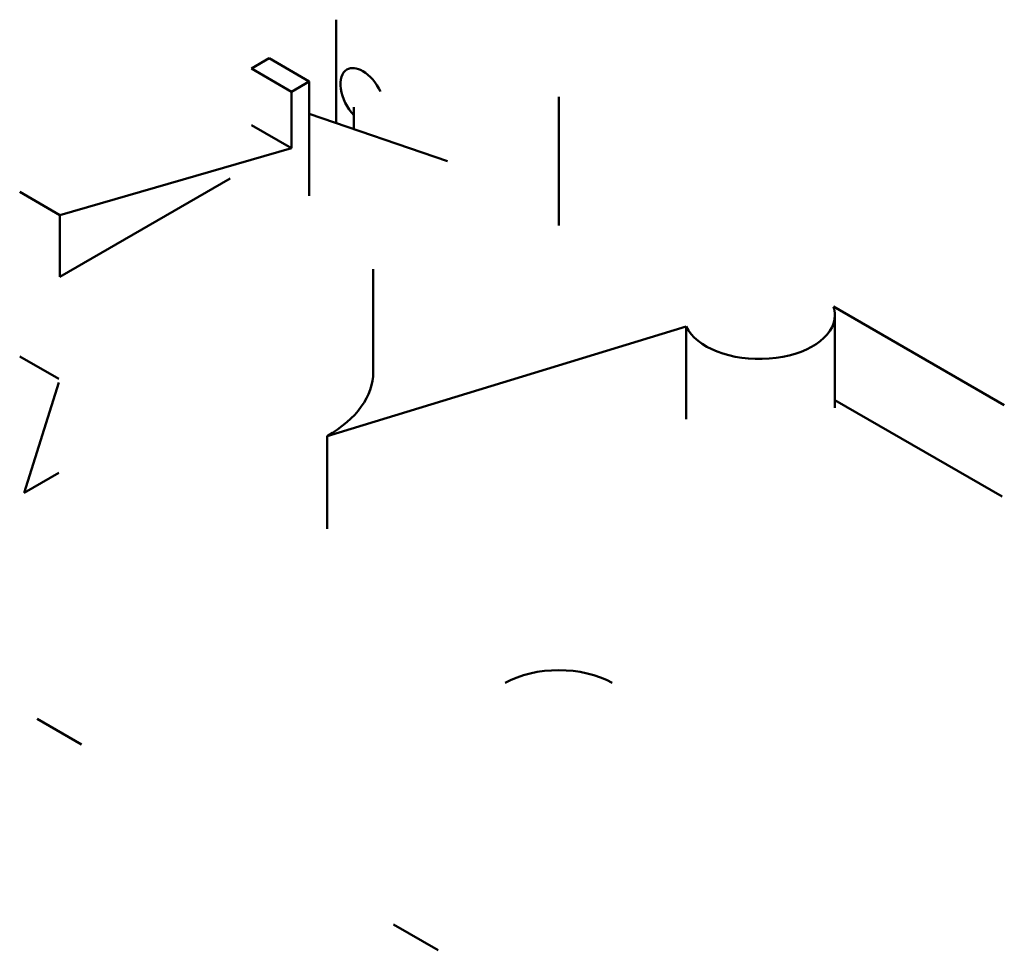
# Model space of a CAD drawing. Units: inches. Extents: x 1911 to 53588, y 1283 to 37932.
# Tile 2 of 2: x 48726 to 53588, y 33334 to 37932. Entities that reach past the tile are written whole.
import ezdxf

# ---------------------------------------------------------------- set-up
doc = ezdxf.new("R2010")
doc.units = ezdxf.units.IN
doc.header["$MEASUREMENT"] = 0
doc.layers.add('M-OUTL', color=7, linetype='Continuous', lineweight=50)

msp = doc.modelspace()

# ---------------------------------------------------------------- linework, layer by layer
at = {"layer": 'M-OUTL'}
for p, q in [((50288.2, 37420.8), (50288.2, 37931.7)), ((49870.2, 37690.4), (49958.2, 37741.2)), ((50156.2, 37626.9), (49958.2, 37741.2)), ((50068.2, 37576.1), (49870.2, 37690.4)), ((50068.2, 37576.1), (50156.2, 37626.9)), ((50156.2, 37626.9), (50156.2, 37061.1)), ((50068.2, 37296.7), (50068.2, 37576.1)), ((51388, 36915.7), (51388, 37550.7)), ((50376.2, 37390.8), (50376.2, 37499.9)), ((50838.1, 37233.2), (50156.2, 37465.9)), ((50068.2, 37296.7), (49870.2, 37411)), ((48924.3, 36966.5), (50068.2, 37296.7)), ((49764.8, 37147), (48924.3, 36661.7)), ((48924.3, 36966.5), (48726.4, 37080.8)), ((48924.3, 36661.7), (48924.3, 36966.5)), ((50472, 36191.8), (50472, 36699.8)), ((52743.8, 36514), (53587.7, 36026.7)), ((52751.2, 36471.2), (52751.2, 36014)), ((50244.2, 35874.3), (52017.3, 36415.4)), ((52017.3, 35958.2), (52017.3, 36415.4)), ((48726.4, 36268), (48918.9, 36156.9)), ((48748.4, 35594.9), (48919.7, 36139.1)), ((52751.2, 36052.5), (53577.3, 35575.5)), ((50244.2, 35417.1), (50244.2, 35874.3)), ((48919.7, 35693.9), (48748.4, 35594.9)), ((49032.3, 34350.2), (48812.3, 34477.2)), ((50792.1, 33334.2), (50572.1, 33461.2))]:
    msp.add_line(p, q, dxfattribs=at)
for centre, major_axis, start_param, end_param in [((50420.1, 37550.7), (77.8, -134.7), 3.141593, 5.08627), ((50420.1, 37550.7), (77.8, -134.7), 2.356194, 3.141593), ((50420.1, 37550.7), (77.8, -134.7), 1.428899, 2.356194), ((52377.9, 36471.2), (373.3, 0), 0, 0.199713), ((52377.9, 36471.2), (373.3, 0), 3.403392, 6.283185), ((49694.2, 36191.8), (777.7, 0), 5.497787, 6.283185), ((51388, 34502.7), (-373.3, 0), 3.926991, 5.497787)]:
    msp.add_ellipse(centre, major_axis=major_axis, ratio=0.57735, start_param=start_param, end_param=end_param, dxfattribs=at)

doc.saveas('drawing.dxf')
